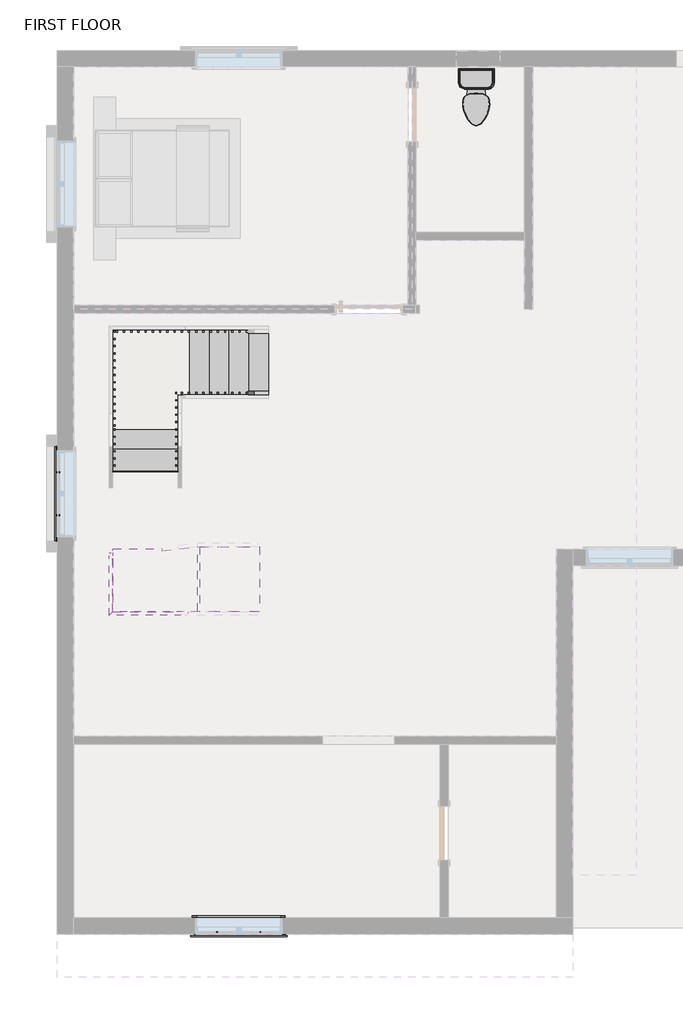
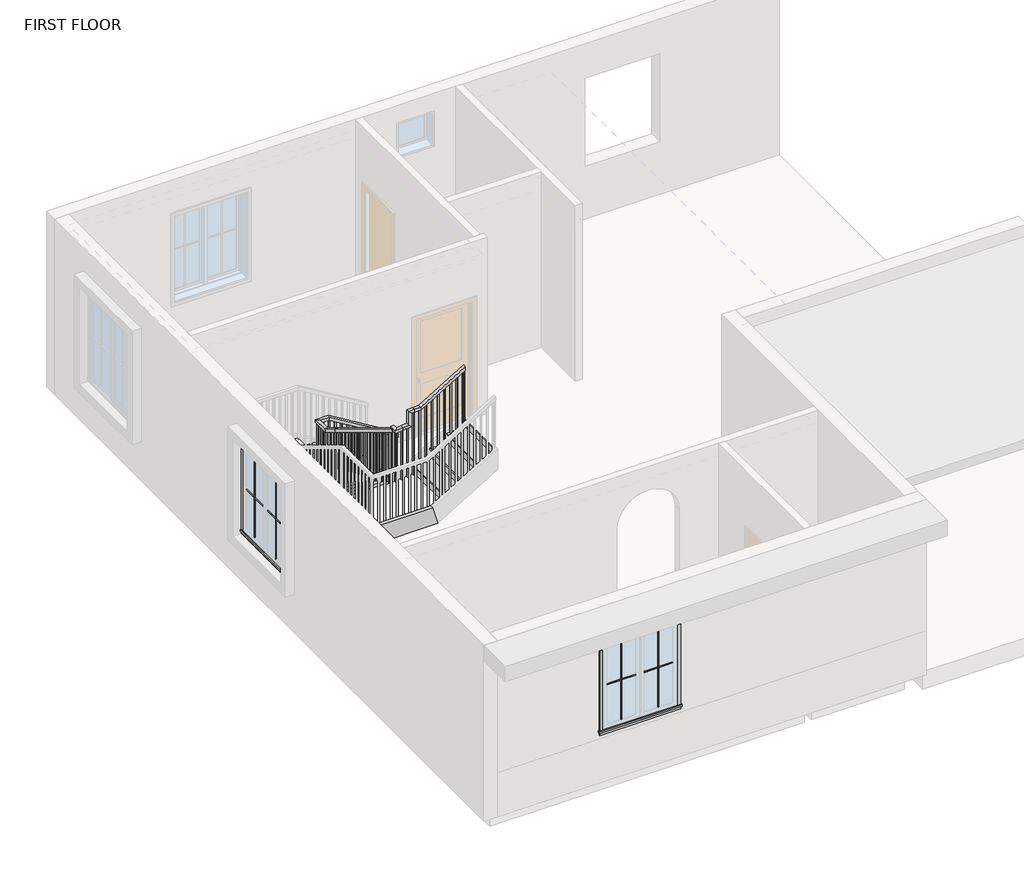
# One storey, part 3 of 4: 7 proxies, 3 stair flights, 2 members, 2 slabs, 1 flow terminal, 1 railing.
"""IFC4 building model written with IfcOpenShell, lengths in millimetres."""

from ifc_helpers import new_model, si_unit, frame, origin, place, context, project, spatial, polyline, outline, extrude, faceted_brep, transform, mapped, element, save
from components import muntin_pattern_2x2_muntin_pattern_2x2_6dad3731, muntin_pattern_2x2_muntin_pattern_2x2_a30a3345, trim_window_exterior_flat_with_sill_92b9b949, trim_window_interior_flat_picture_frame_3bb882cf, toilet_domestic_3d_toilet_domestic_3d_ba6479b0, toilet_domestic_3d_toilet_domestic_3d_30431060, non_monolithic_landing_30da2899, non_monolithic_landing_a4a5f0de, stair_flight_f80b6bc8, stair_flight_52aa9efe, stair_flight_812e3324

model = new_model("IFC4")

# Units and contexts
model_context = context("Model", 3, world=origin())
ifc_project = project(units=[si_unit("LENGTHUNIT", "METRE", prefix="MILLI")], contexts=[model_context])

# Site, building, storey
site = spatial("IfcSite", under=ifc_project)
building = spatial("IfcBuilding", under=site)
storey = spatial("IfcBuildingStorey", under=building, Name="FIRST FLOOR", Elevation=3352.8)

# Proxies
placement = place(None, origin())
muntin_pattern_2x2_muntin_pattern_2x2_shape = muntin_pattern_2x2_muntin_pattern_2x2_6dad3731(model_context)
element("IfcBuildingElementProxy", 1, Name="Muntin Pattern_2x2 : Muntin Pattern_2x2", ObjectType="Muntin Pattern_2x2 : Muntin Pattern_2x2", at=placement, inside=storey, context=model_context, shape_type="MappedRepresentation", body=[
    mapped(muntin_pattern_2x2_muntin_pattern_2x2_shape, transform((-9193.7461008, -7440.4594117, 4337.05), x_axis=(-1.0, 0.0, 0.0), y_axis=(0.0, -1.0, 0.0), z_axis=(0.0, 0.0, 1.0))),
])
element("IfcBuildingElementProxy", 2, Name="Muntin Pattern_2x2 : Muntin Pattern_2x2", ObjectType="Muntin Pattern_2x2 : Muntin Pattern_2x2", at=placement, inside=storey, context=model_context, shape_type="MappedRepresentation", body=[
    mapped(muntin_pattern_2x2_muntin_pattern_2x2_shape, transform((-12040.1336008, -1561.9469117, 4337.05), x_axis=(0.0, 1.0, 0.0), y_axis=(-1.0, 0.0, 0.0), z_axis=(0.0, 0.0, 1.0))),
])
muntin_pattern_2x2_muntin_pattern_2x2_2_shape = muntin_pattern_2x2_muntin_pattern_2x2_a30a3345(model_context)
element("IfcBuildingElementProxy", 3, Name="Muntin Pattern_2x2 : Muntin Pattern_2x2", ObjectType="Muntin Pattern_2x2 : Muntin Pattern_2x2", at=placement, inside=storey, context=model_context, shape_type="MappedRepresentation", body=[
    mapped(muntin_pattern_2x2_muntin_pattern_2x2_2_shape, transform((-9800.1711008, -7440.4594117, 4337.05), x_axis=(1.0, 0.0, 0.0), y_axis=(0.0, 1.0, 0.0), z_axis=(0.0, 0.0, 1.0))),
])
element("IfcBuildingElementProxy", 4, Name="Muntin Pattern_2x2 : Muntin Pattern_2x2", ObjectType="Muntin Pattern_2x2 : Muntin Pattern_2x2", at=placement, inside=storey, context=model_context, shape_type="MappedRepresentation", body=[
    mapped(muntin_pattern_2x2_muntin_pattern_2x2_2_shape, transform((-12040.1336008, -955.5219117, 4337.05), x_axis=(0.0, -1.0, 0.0), y_axis=(1.0, 0.0, 0.0), z_axis=(0.0, 0.0, 1.0))),
])
trim_window_exterior_flat_with_sill_shape = trim_window_exterior_flat_with_sill_92b9b949(model_context)
element("IfcBuildingElementProxy", 5, Name="Trim-Window-Exterior-Flat : with Sill", ObjectType="Trim-Window-Exterior-Flat : with Sill", at=placement, inside=storey, context=model_context, shape_type="MappedRepresentation", body=[
    mapped(trim_window_exterior_flat_with_sill_shape, transform((-9496.9586008, -7449.9844117, 5791.2), x_axis=(1.0, 0.0, 0.0), y_axis=(0.0, 0.0, 1.0), z_axis=(0.0, -1.0, 0.0))),
])
element("IfcBuildingElementProxy", 6, Name="Trim-Window-Exterior-Flat : with Sill", ObjectType="Trim-Window-Exterior-Flat : with Sill", at=placement, inside=storey, context=model_context, shape_type="MappedRepresentation", body=[
    mapped(trim_window_exterior_flat_with_sill_shape, transform((-12049.6586008, -1258.7344117, 5791.2), x_axis=(0.0, -1.0, 0.0), y_axis=(0.0, 0.0, 1.0), z_axis=(-1.0, 0.0, 0.0))),
])
trim_window_interior_flat_picture_frame_shape = trim_window_interior_flat_picture_frame_3bb882cf(model_context)
element("IfcBuildingElementProxy", 7, Name="Trim-Window-Interior-Flat : Picture Frame", ObjectType="Trim-Window-Interior-Flat : Picture Frame", at=placement, inside=storey, context=model_context, shape_type="MappedRepresentation", body=[
    mapped(trim_window_interior_flat_picture_frame_shape, transform((-9496.9586008, -7221.3844117, 5791.2), x_axis=(-1.0, 0.0, 0.0), y_axis=(0.0, 0.0, 1.0), z_axis=(0.0, 1.0, 0.0))),
])

# Flow terminal
toilet_domestic_3d_toilet_domestic_3d_shape = toilet_domestic_3d_toilet_domestic_3d_ba6479b0(model_context)
toilet_domestic_3d_toilet_domestic_3d_2_shape = toilet_domestic_3d_toilet_domestic_3d_30431060(model_context)
element("IfcFlowTerminal", 8, ObjectType="Toilet-Domestic-3D : Toilet-Domestic-3D", at=placement, inside=storey, context=model_context, shape_type="MappedRepresentation", body=[
    mapped(toilet_domestic_3d_toilet_domestic_3d_shape, transform((-6156.8586008, 4221.3155883, 3352.8), x_axis=(1.0, 0.0, 0.0), y_axis=(0.0, 1.0, 0.0), z_axis=(0.0, 0.0, 1.0))),
    mapped(toilet_domestic_3d_toilet_domestic_3d_2_shape, transform((-6156.8586008, 4221.3155883, 3352.8), x_axis=(1.0, 0.0, 0.0), y_axis=(0.0, 1.0, 0.0), z_axis=(0.0, 0.0, 1.0))),
])

# Members
element("IfcMember", 9, ObjectType="Stringer - 2\" Width", at=placement, inside=storey, context=model_context, shape_type="Brep", body=[
    faceted_brep([(-11268.1522729, -2087.9404207, 5461.0), (-11318.9522729, -2087.9404207, 5461.0), (-11318.9522729, -2966.8844117, 5461.0), (-11268.1522729, -2916.0844117, 5461.0), (-11268.1522729, -2173.0948772, 5156.2), (-11268.1522729, -2916.0844117, 5156.2), (-11318.9522729, -2173.0948772, 5156.2), (-11318.9522729, -2966.8844117, 5156.2)], [[[0, 1, 2, 3]], [[4, 0, 3, 5]], [[6, 4, 5, 7]], [[1, 6, 7, 2]], [[1, 0, 4, 6]], [[2, 7, 5, 3]]]),
])
element("IfcMember", 10, ObjectType="Stringer - 2\" Width", at=placement, inside=storey, context=model_context, shape_type="Brep", body=[
    faceted_brep([(-11268.1522729, -2916.0844117, 5461.0), (-11318.9522729, -2966.8844117, 5461.0), (-10298.6112176, -2966.8844117, 5461.0), (-10298.6112176, -2916.0844117, 5461.0), (-11268.1522729, -2916.0844117, 5156.2), (-10213.4567611, -2916.0844117, 5156.2), (-11318.9522729, -2966.8844117, 5156.2), (-10213.4567611, -2966.8844117, 5156.2)], [[[0, 1, 2, 3]], [[4, 0, 3, 5]], [[6, 4, 5, 7]], [[1, 6, 7, 2]], [[1, 0, 4, 6]], [[2, 7, 5, 3]]]),
])

# Railing
element("IfcRailing", 11, ObjectType="Handrail - Rectangular", at=placement, inside=storey, context=model_context, shape_type="SolidModel", body=[
    faceted_brep([(-9079.7156858, 130.7115003, 4436.5333333), (-9079.7156858, 130.7115003, 4377.1318731), (-9079.7156858, 181.5115003, 4377.1318731), (-9079.7156858, 181.5115003, 4436.5333333), (-10197.3156858, 130.7115003, 5113.8666667), (-10211.5080953, 130.7115003, 5063.0666667), (-10211.5080953, 181.5115003, 5063.0666667), (-10197.3156858, 181.5115003, 5113.8666667), (-10353.7522729, 130.7115003, 5113.8666667), (-10353.7522729, 130.7115003, 5063.0666667), (-10404.5522729, 181.5115003, 5063.0666667), (-10404.5522729, 181.5115003, 5113.8666667), (-10353.7522729, -76.9993654, 5113.8666667), (-10353.7522729, -91.1917748, 5063.0666667), (-10404.5522729, -91.1917748, 5063.0666667), (-10404.5522729, -76.9993654, 5113.8666667), (-10353.7522729, -356.3993654, 5283.2), (-10353.7522729, -382.7290926, 5239.7559502), (-10404.5522729, -382.7290926, 5239.7559502), (-10404.5522729, -356.3993654, 5283.2), (-10353.7522729, -1959.5850154, 6254.8276667), (-10353.7522729, -2010.3850154, 6226.2140852), (-10404.5522729, -2010.3850154, 6226.2140852), (-10404.5522729, -1959.5850154, 6254.8276667), (-10353.7522729, -1959.5850154, 6299.2), (-10353.7522729, -2010.3850154, 6248.4), (-10404.5522729, -2010.3850154, 6248.4), (-10404.5522729, -1959.5850154, 6299.2), (-10353.7522729, -2032.7993654, 6299.2), (-10353.7522729, -2032.7993654, 6248.4), (-10404.5522729, -2089.5706654, 6248.4), (-10404.5522729, -2089.5706654, 6299.2), (-10280.987739, -2024.6960544, 6299.2), (-10280.987739, -2024.6960544, 6248.4), (-10275.3652319, -2075.1839481, 6248.4), (-10275.3652319, -2075.1839481, 6299.2), (-10176.7293559, -2013.085479, 6299.2), (-10126.2414621, -2007.4629719, 6248.4), (-10120.6189551, -2057.9508656, 6248.4), (-10171.1068488, -2063.5733727, 6299.2), (-10176.7293559, -2013.085479, 6530.9636109), (-10126.2414621, -2007.4629719, 6480.1636109), (-10120.6189551, -2057.9508656, 6480.1636109), (-10171.1068488, -2063.5733727, 6530.9636109), (-10074.3522729, -2001.6844117, 6530.9636109), (-10074.3522729, -2001.6844117, 6480.1636109), (-10071.5323568, -2052.4844117, 6480.1636109), (-10071.5323568, -2052.4844117, 6530.9636109), (-9971.3423149, -2001.6844117, 6530.9636109), (-9957.1499054, -2001.6844117, 6480.1636109), (-9957.1499054, -2052.4844117, 6480.1636109), (-9971.3423149, -2052.4844117, 6530.9636109), (-9236.1522729, -2001.6844117, 6976.5333333), (-9236.1522729, -2052.4844117, 6976.5333333), (-9236.1522729, -2052.4844117, 6917.1318731), (-9236.1522729, -2001.6844117, 6917.1318731)], [[[0, 1, 2, 3]], [[1, 0, 4, 5]], [[2, 1, 5, 6]], [[3, 2, 6, 7]], [[0, 3, 7, 4]], [[5, 4, 8, 9]], [[6, 5, 9, 10]], [[7, 6, 10, 11]], [[4, 7, 11, 8]], [[9, 8, 12, 13]], [[10, 9, 13, 14]], [[11, 10, 14, 15]], [[8, 11, 15, 12]], [[13, 12, 16, 17]], [[14, 13, 17, 18]], [[15, 14, 18, 19]], [[12, 15, 19, 16]], [[17, 16, 20, 21]], [[18, 17, 21, 22]], [[19, 18, 22, 23]], [[16, 19, 23, 20]], [[21, 20, 24, 25]], [[22, 21, 25, 26]], [[23, 22, 26, 27]], [[20, 23, 27, 24]], [[25, 24, 28, 29]], [[26, 25, 29, 30]], [[27, 26, 30, 31]], [[24, 27, 31, 28]], [[29, 28, 32, 33]], [[30, 29, 33, 34]], [[31, 30, 34, 35]], [[28, 31, 35, 32]], [[33, 32, 36, 37]], [[34, 33, 37, 38]], [[35, 34, 38, 39]], [[32, 35, 39, 36]], [[37, 36, 40, 41]], [[38, 37, 41, 42]], [[39, 38, 42, 43]], [[36, 39, 43, 40]], [[41, 40, 44, 45]], [[42, 41, 45, 46]], [[43, 42, 46, 47]], [[40, 43, 47, 44]], [[45, 44, 48, 49]], [[46, 45, 49, 50]], [[47, 46, 50, 51]], [[44, 47, 51, 48]], [[52, 53, 54, 55]], [[49, 48, 52, 55]], [[50, 49, 55, 54]], [[51, 50, 54, 53]], [[48, 51, 53, 52]]]),
    extrude(outline(polyline([(6896.8197264, -9269.6673149), (5892.8, -9269.6673149), (5892.8, -9250.6173149), (6908.365181, -9250.6173149), (6896.8197264, -9269.6673149)])), frame((0.0, -2036.6094117, 0.0), z_axis=(0.0, 1.0, 0.0), x_axis=(0.0, 0.0, 1.0)), (0.0, 0.0, 1.0), 19.05),
    extrude(outline(polyline([(6835.2439689, -9371.2673149), (5892.8, -9371.2673149), (5892.8, -9352.2173149), (6846.7894234, -9352.2173149), (6835.2439689, -9371.2673149)])), frame((0.0, -2036.6094117, 0.0), z_axis=(0.0, 1.0, 0.0), x_axis=(0.0, 0.0, 1.0)), (0.0, 0.0, 1.0), 19.05),
    extrude(outline(polyline([(6773.6682113, -9472.8673149), (5892.8, -9472.8673149), (5892.8, -9453.8173149), (6785.2136658, -9453.8173149), (6773.6682113, -9472.8673149)])), frame((0.0, -2036.6094117, 0.0), z_axis=(0.0, 1.0, 0.0), x_axis=(0.0, 0.0, 1.0)), (0.0, 0.0, 1.0), 19.05),
    extrude(outline(polyline([(6712.0924537, -9574.4673149), (5723.4666667, -9574.4673149), (5723.4666667, -9555.4173149), (6723.6379083, -9555.4173149), (6712.0924537, -9574.4673149)])), frame((0.0, -2036.6094117, 0.0), z_axis=(0.0, 1.0, 0.0), x_axis=(0.0, 0.0, 1.0)), (0.0, 0.0, 1.0), 19.05),
    extrude(outline(polyline([(6650.5166961, -9676.0673149), (5723.4666667, -9676.0673149), (5723.4666667, -9657.0173149), (6662.0621507, -9657.0173149), (6650.5166961, -9676.0673149)])), frame((0.0, -2036.6094117, 0.0), z_axis=(0.0, 1.0, 0.0), x_axis=(0.0, 0.0, 1.0)), (0.0, 0.0, 1.0), 19.05),
    extrude(outline(polyline([(6588.9409386, -9777.6673149), (5723.4666667, -9777.6673149), (5723.4666667, -9758.6173149), (6600.4863931, -9758.6173149), (6588.9409386, -9777.6673149)])), frame((0.0, -2036.6094117, 0.0), z_axis=(0.0, 1.0, 0.0), x_axis=(0.0, 0.0, 1.0)), (0.0, 0.0, 1.0), 19.05),
    extrude(outline(polyline([(6527.365181, -9879.2673149), (5554.1333333, -9879.2673149), (5554.1333333, -9860.2173149), (6538.9106355, -9860.2173149), (6527.365181, -9879.2673149)])), frame((0.0, -2036.6094117, 0.0), z_axis=(0.0, 1.0, 0.0), x_axis=(0.0, 0.0, 1.0)), (0.0, 0.0, 1.0), 19.05),
    extrude(outline(polyline([(6465.7894234, -9980.8673149), (5554.1333333, -9980.8673149), (5554.1333333, -9961.8173149), (6477.334878, -9961.8173149), (6465.7894234, -9980.8673149)])), frame((0.0, -2036.6094117, 0.0), z_axis=(0.0, 1.0, 0.0), x_axis=(0.0, 0.0, 1.0)), (0.0, 0.0, 1.0), 19.05),
    extrude(outline(polyline([(-10086.7456106, -2019.0377129), (-10067.8126505, -2016.9292728), (-10065.7042103, -2035.8622329), (-10084.6371705, -2037.9706731), (-10086.7456106, -2019.0377129)])), frame((0.0, 0.0, 5384.8), z_axis=(0.0, 0.0, 1.0), x_axis=(1.0, 0.0, 0.0)), (0.0, 0.0, 1.0), 1095.3636109),
    extrude(outline(polyline([(-10187.7213981, -2030.2827271), (-10168.7884379, -2028.1742869), (-10166.6799978, -2047.1072471), (-10185.6129579, -2049.2156872), (-10187.7213981, -2030.2827271)])), frame((0.0, 0.0, 5384.8), z_axis=(0.0, 0.0, 1.0), x_axis=(1.0, 0.0, 0.0)), (0.0, 0.0, 1.0), 863.6),
    extrude(outline(polyline([(-10288.6971856, -2041.5277412), (-10269.7642254, -2039.4193011), (-10267.6557853, -2058.3522612), (-10286.5887454, -2060.4607014), (-10288.6971856, -2041.5277412)])), frame((0.0, 0.0, 5384.8), z_axis=(0.0, 0.0, 1.0), x_axis=(1.0, 0.0, 0.0)), (0.0, 0.0, 1.0), 863.6),
    extrude(outline(polyline([(-10369.6272729, -1972.4743654), (-10369.6272729, -1991.5243654), (-10388.6772729, -1991.5243654), (-10388.6772729, -1972.4743654), (-10369.6272729, -1972.4743654)])), frame((0.0, 0.0, 5215.4666667), z_axis=(0.0, 0.0, 1.0), x_axis=(1.0, 0.0, 0.0)), (0.0, 0.0, 1.0), 1032.9333333),
    extrude(outline(polyline([(-1870.8743654, 6141.6621761), (-1870.8743654, 5215.4666667), (-1889.9243654, 5215.4666667), (-1889.9243654, 6153.2076307), (-1870.8743654, 6141.6621761)])), frame((-10388.6772729, 0.0, 0.0), z_axis=(1.0, 0.0, 0.0), x_axis=(0.0, 1.0, 0.0)), (0.0, 0.0, 1.0), 19.05),
    extrude(outline(polyline([(-1769.2743654, 6080.0864185), (-1769.2743654, 5215.4666667), (-1788.3243654, 5215.4666667), (-1788.3243654, 6091.6318731), (-1769.2743654, 6080.0864185)])), frame((-10388.6772729, 0.0, 0.0), z_axis=(1.0, 0.0, 0.0), x_axis=(0.0, 1.0, 0.0)), (0.0, 0.0, 1.0), 19.05),
    extrude(outline(polyline([(-1667.6743654, 6018.510661), (-1667.6743654, 5046.1333333), (-1686.7243654, 5046.1333333), (-1686.7243654, 6030.0561155), (-1667.6743654, 6018.510661)])), frame((-10388.6772729, 0.0, 0.0), z_axis=(1.0, 0.0, 0.0), x_axis=(0.0, 1.0, 0.0)), (0.0, 0.0, 1.0), 19.05),
    extrude(outline(polyline([(-1566.0743654, 5956.9349034), (-1566.0743654, 5046.1333333), (-1585.1243654, 5046.1333333), (-1585.1243654, 5968.4803579), (-1566.0743654, 5956.9349034)])), frame((-10388.6772729, 0.0, 0.0), z_axis=(1.0, 0.0, 0.0), x_axis=(0.0, 1.0, 0.0)), (0.0, 0.0, 1.0), 19.05),
    extrude(outline(polyline([(-1464.4743654, 5895.3591458), (-1464.4743654, 5046.1333333), (-1483.5243654, 5046.1333333), (-1483.5243654, 5906.9046004), (-1464.4743654, 5895.3591458)])), frame((-10388.6772729, 0.0, 0.0), z_axis=(1.0, 0.0, 0.0), x_axis=(0.0, 1.0, 0.0)), (0.0, 0.0, 1.0), 19.05),
    extrude(outline(polyline([(-1362.8743654, 5833.7833882), (-1362.8743654, 4876.8), (-1381.9243654, 4876.8), (-1381.9243654, 5845.3288428), (-1362.8743654, 5833.7833882)])), frame((-10388.6772729, 0.0, 0.0), z_axis=(1.0, 0.0, 0.0), x_axis=(0.0, 1.0, 0.0)), (0.0, 0.0, 1.0), 19.05),
    extrude(outline(polyline([(-1261.2743654, 5772.2076307), (-1261.2743654, 4876.8), (-1280.3243654, 4876.8), (-1280.3243654, 5783.7530852), (-1261.2743654, 5772.2076307)])), frame((-10388.6772729, 0.0, 0.0), z_axis=(1.0, 0.0, 0.0), x_axis=(0.0, 1.0, 0.0)), (0.0, 0.0, 1.0), 19.05),
    extrude(outline(polyline([(-1159.6743654, 5710.6318731), (-1159.6743654, 4707.4666667), (-1178.7243654, 4707.4666667), (-1178.7243654, 5722.1773276), (-1159.6743654, 5710.6318731)])), frame((-10388.6772729, 0.0, 0.0), z_axis=(1.0, 0.0, 0.0), x_axis=(0.0, 1.0, 0.0)), (0.0, 0.0, 1.0), 19.05),
    extrude(outline(polyline([(-1058.0743654, 5649.0561155), (-1058.0743654, 4707.4666667), (-1077.1243654, 4707.4666667), (-1077.1243654, 5660.60157), (-1058.0743654, 5649.0561155)])), frame((-10388.6772729, 0.0, 0.0), z_axis=(1.0, 0.0, 0.0), x_axis=(0.0, 1.0, 0.0)), (0.0, 0.0, 1.0), 19.05),
    extrude(outline(polyline([(-956.4743654, 5587.4803579), (-956.4743654, 4707.4666667), (-975.5243654, 4707.4666667), (-975.5243654, 5599.0258125), (-956.4743654, 5587.4803579)])), frame((-10388.6772729, 0.0, 0.0), z_axis=(1.0, 0.0, 0.0), x_axis=(0.0, 1.0, 0.0)), (0.0, 0.0, 1.0), 19.05),
    extrude(outline(polyline([(-854.8743654, 5525.9046004), (-854.8743654, 4538.1333333), (-873.9243654, 4538.1333333), (-873.9243654, 5537.4500549), (-854.8743654, 5525.9046004)])), frame((-10388.6772729, 0.0, 0.0), z_axis=(1.0, 0.0, 0.0), x_axis=(0.0, 1.0, 0.0)), (0.0, 0.0, 1.0), 19.05),
    extrude(outline(polyline([(-753.2743654, 5464.3288428), (-753.2743654, 4538.1333333), (-772.3243654, 4538.1333333), (-772.3243654, 5475.8742973), (-753.2743654, 5464.3288428)])), frame((-10388.6772729, 0.0, 0.0), z_axis=(1.0, 0.0, 0.0), x_axis=(0.0, 1.0, 0.0)), (0.0, 0.0, 1.0), 19.05),
    extrude(outline(polyline([(-651.6743654, 5402.7530852), (-651.6743654, 4538.1333333), (-670.7243654, 4538.1333333), (-670.7243654, 5414.2985397), (-651.6743654, 5402.7530852)])), frame((-10388.6772729, 0.0, 0.0), z_axis=(1.0, 0.0, 0.0), x_axis=(0.0, 1.0, 0.0)), (0.0, 0.0, 1.0), 19.05),
    extrude(outline(polyline([(-550.0743654, 5341.1773276), (-550.0743654, 4368.8), (-569.1243654, 4368.8), (-569.1243654, 5352.7227822), (-550.0743654, 5341.1773276)])), frame((-10388.6772729, 0.0, 0.0), z_axis=(1.0, 0.0, 0.0), x_axis=(0.0, 1.0, 0.0)), (0.0, 0.0, 1.0), 19.05),
    extrude(outline(polyline([(-448.4743654, 5279.60157), (-448.4743654, 4368.8), (-467.5243654, 4368.8), (-467.5243654, 5291.1470246), (-448.4743654, 5279.60157)])), frame((-10388.6772729, 0.0, 0.0), z_axis=(1.0, 0.0, 0.0), x_axis=(0.0, 1.0, 0.0)), (0.0, 0.0, 1.0), 19.05),
    extrude(outline(polyline([(-342.3634997, 5215.2919545), (-342.3634997, 4199.4666667), (-361.4134997, 4199.4666667), (-361.4134997, 5226.837409), (-342.3634997, 5215.2919545)])), frame((-10388.6772729, 0.0, 0.0), z_axis=(1.0, 0.0, 0.0), x_axis=(0.0, 1.0, 0.0)), (0.0, 0.0, 1.0), 19.05),
    extrude(outline(polyline([(-240.7634997, 5153.7161969), (-240.7634997, 4199.4666667), (-259.8134997, 4199.4666667), (-259.8134997, 5165.2616515), (-240.7634997, 5153.7161969)])), frame((-10388.6772729, 0.0, 0.0), z_axis=(1.0, 0.0, 0.0), x_axis=(0.0, 1.0, 0.0)), (0.0, 0.0, 1.0), 19.05),
    extrude(outline(polyline([(-139.1634997, 5092.1404393), (-139.1634997, 4199.4666667), (-158.2134997, 4199.4666667), (-158.2134997, 5103.6858939), (-139.1634997, 5092.1404393)])), frame((-10388.6772729, 0.0, 0.0), z_axis=(1.0, 0.0, 0.0), x_axis=(0.0, 1.0, 0.0)), (0.0, 0.0, 1.0), 19.05),
    extrude(outline(polyline([(-10369.6272729, -37.5634997), (-10369.6272729, -56.6134997), (-10388.6772729, -56.6134997), (-10388.6772729, -37.5634997), (-10369.6272729, -37.5634997)])), frame((0.0, 0.0, 4199.4666667), z_axis=(0.0, 0.0, 1.0), x_axis=(1.0, 0.0, 0.0)), (0.0, 0.0, 1.0), 863.6),
    extrude(outline(polyline([(-10369.6272729, 64.0365003), (-10369.6272729, 44.9865003), (-10388.6772729, 44.9865003), (-10388.6772729, 64.0365003), (-10369.6272729, 64.0365003)])), frame((0.0, 0.0, 4199.4666667), z_axis=(0.0, 0.0, 1.0), x_axis=(1.0, 0.0, 0.0)), (0.0, 0.0, 1.0), 863.6),
    extrude(outline(polyline([(-10289.3906858, 146.5865003), (-10308.4406858, 146.5865003), (-10308.4406858, 165.6365003), (-10289.3906858, 165.6365003), (-10289.3906858, 146.5865003)])), frame((0.0, 0.0, 4199.4666667), z_axis=(0.0, 0.0, 1.0), x_axis=(1.0, 0.0, 0.0)), (0.0, 0.0, 1.0), 863.6),
    extrude(outline(polyline([(4998.6621761, -10105.2406858), (4030.1333333, -10105.2406858), (4030.1333333, -10086.1906858), (4987.1167216, -10086.1906858), (4998.6621761, -10105.2406858)])), frame((0.0, 146.5865003, 0.0), z_axis=(0.0, 1.0, 0.0), x_axis=(0.0, 0.0, 1.0)), (0.0, 0.0, 1.0), 19.05),
    extrude(outline(polyline([(4937.0864185, -10003.6406858), (4030.1333333, -10003.6406858), (4030.1333333, -9984.5906858), (4925.540964, -9984.5906858), (4937.0864185, -10003.6406858)])), frame((0.0, 146.5865003, 0.0), z_axis=(0.0, 1.0, 0.0), x_axis=(0.0, 0.0, 1.0)), (0.0, 0.0, 1.0), 19.05),
    extrude(outline(polyline([(4875.510661, -9902.0406858), (3860.8, -9902.0406858), (3860.8, -9882.9906858), (4863.9652064, -9882.9906858), (4875.510661, -9902.0406858)])), frame((0.0, 146.5865003, 0.0), z_axis=(0.0, 1.0, 0.0), x_axis=(0.0, 0.0, 1.0)), (0.0, 0.0, 1.0), 19.05),
    extrude(outline(polyline([(4813.9349034, -9800.4406858), (3860.8, -9800.4406858), (3860.8, -9781.3906858), (4802.3894488, -9781.3906858), (4813.9349034, -9800.4406858)])), frame((0.0, 146.5865003, 0.0), z_axis=(0.0, 1.0, 0.0), x_axis=(0.0, 0.0, 1.0)), (0.0, 0.0, 1.0), 19.05),
    extrude(outline(polyline([(4752.3591458, -9698.8406858), (3860.8, -9698.8406858), (3860.8, -9679.7906858), (4740.8136913, -9679.7906858), (4752.3591458, -9698.8406858)])), frame((0.0, 146.5865003, 0.0), z_axis=(0.0, 1.0, 0.0), x_axis=(0.0, 0.0, 1.0)), (0.0, 0.0, 1.0), 19.05),
    extrude(outline(polyline([(4690.7833882, -9597.2406858), (3691.4666667, -9597.2406858), (3691.4666667, -9578.1906858), (4679.2379337, -9578.1906858), (4690.7833882, -9597.2406858)])), frame((0.0, 146.5865003, 0.0), z_axis=(0.0, 1.0, 0.0), x_axis=(0.0, 0.0, 1.0)), (0.0, 0.0, 1.0), 19.05),
    extrude(outline(polyline([(4629.2076307, -9495.6406858), (3691.4666667, -9495.6406858), (3691.4666667, -9476.5906858), (4617.6621761, -9476.5906858), (4629.2076307, -9495.6406858)])), frame((0.0, 146.5865003, 0.0), z_axis=(0.0, 1.0, 0.0), x_axis=(0.0, 0.0, 1.0)), (0.0, 0.0, 1.0), 19.05),
    extrude(outline(polyline([(4567.6318731, -9394.0406858), (3691.4666667, -9394.0406858), (3691.4666667, -9374.9906858), (4556.0864185, -9374.9906858), (4567.6318731, -9394.0406858)])), frame((0.0, 146.5865003, 0.0), z_axis=(0.0, 1.0, 0.0), x_axis=(0.0, 0.0, 1.0)), (0.0, 0.0, 1.0), 19.05),
    extrude(outline(polyline([(4506.0561155, -9292.4406858), (3522.1333333, -9292.4406858), (3522.1333333, -9273.3906858), (4494.510661, -9273.3906858), (4506.0561155, -9292.4406858)])), frame((0.0, 146.5865003, 0.0), z_axis=(0.0, 1.0, 0.0), x_axis=(0.0, 0.0, 1.0)), (0.0, 0.0, 1.0), 19.05),
    extrude(outline(polyline([(4444.4803579, -9190.8406858), (3522.1333333, -9190.8406858), (3522.1333333, -9171.7906858), (4432.9349034, -9171.7906858), (4444.4803579, -9190.8406858)])), frame((0.0, 146.5865003, 0.0), z_axis=(0.0, 1.0, 0.0), x_axis=(0.0, 0.0, 1.0)), (0.0, 0.0, 1.0), 19.05),
    extrude(outline(polyline([(-10083.463015, -2018.6721517), (-10064.5300549, -2016.5637115), (-10062.4216147, -2035.4966717), (-10081.3545749, -2037.6051118), (-10083.463015, -2018.6721517)])), frame((0.0, 0.0, 5384.8), z_axis=(0.0, 0.0, 1.0), x_axis=(1.0, 0.0, 0.0)), (0.0, 0.0, 1.0), 1095.3636109),
    extrude(outline(polyline([(-10369.6272729, -2051.6600154), (-10369.6272729, -2070.7100154), (-10388.6772729, -2070.7100154), (-10388.6772729, -2051.6600154), (-10369.6272729, -2051.6600154)])), frame((0.0, 0.0, 5384.8), z_axis=(0.0, 0.0, 1.0), x_axis=(1.0, 0.0, 0.0)), (0.0, 0.0, 1.0), 863.6),
    extrude(outline(polyline([(-346.8743654, 5218.0258125), (-346.8743654, 4199.4666667), (-365.9243654, 4199.4666667), (-365.9243654, 5229.571267), (-346.8743654, 5218.0258125)])), frame((-10388.6772729, 0.0, 0.0), z_axis=(1.0, 0.0, 0.0), x_axis=(0.0, 1.0, 0.0)), (0.0, 0.0, 1.0), 19.05),
    extrude(outline(polyline([(-10369.6272729, 146.5865003), (-10388.6772729, 146.5865003), (-10388.6772729, 165.6365003), (-10369.6272729, 165.6365003), (-10369.6272729, 146.5865003)])), frame((0.0, 0.0, 4199.4666667), z_axis=(0.0, 0.0, 1.0), x_axis=(1.0, 0.0, 0.0)), (0.0, 0.0, 1.0), 863.6),
    extrude(outline(polyline([(5060.2379337, -10206.8406858), (4199.4666667, -10206.8406858), (4199.4666667, -10187.7906858), (5048.6924791, -10187.7906858), (5060.2379337, -10206.8406858)])), frame((0.0, 146.5865003, 0.0), z_axis=(0.0, 1.0, 0.0), x_axis=(0.0, 0.0, 1.0)), (0.0, 0.0, 1.0), 19.05),
    extrude(outline(polyline([(6905.5864185, -9255.2022729), (5892.8, -9255.2022729), (5892.8, -9236.1522729), (6917.1318731, -9236.1522729), (6905.5864185, -9255.2022729)])), frame((0.0, -2036.6094117, 0.0), z_axis=(0.0, 1.0, 0.0), x_axis=(0.0, 0.0, 1.0)), (0.0, 0.0, 1.0), 19.05),
    extrude(outline(polyline([(4388.6773276, -9098.7656858), (3522.1333333, -9098.7656858), (3522.1333333, -9079.7156858), (4377.1318731, -9079.7156858), (4388.6773276, -9098.7656858)])), frame((0.0, 146.5865003, 0.0), z_axis=(0.0, 1.0, 0.0), x_axis=(0.0, 0.0, 1.0)), (0.0, 0.0, 1.0), 19.05),
])

# Slabs
non_monolithic_landing_shape = non_monolithic_landing_30da2899(model_context)
element("IfcSlab", 12, ObjectType="Non-Monolithic Landing", at=placement, inside=storey, context=model_context, shape_type="MappedRepresentation", body=[
    mapped(non_monolithic_landing_shape, transform((0.0, 0.0, 0.0), x_axis=(1.0, 0.0, 0.0), y_axis=(0.0, 1.0, 0.0), z_axis=(0.0, 0.0, 1.0))),
])
non_monolithic_landing_2_shape = non_monolithic_landing_a4a5f0de(model_context)
element("IfcSlab", 13, ObjectType="Non-Monolithic Landing", at=placement, inside=storey, context=model_context, shape_type="MappedRepresentation", body=[
    mapped(non_monolithic_landing_2_shape, transform((0.0, 0.0, 0.0), x_axis=(1.0, 0.0, 0.0), y_axis=(0.0, 1.0, 0.0), z_axis=(0.0, 0.0, 1.0))),
])

# Stair flights
stair_flight_shape = stair_flight_f80b6bc8(model_context)
element("IfcStairFlight", 14, ObjectType="2\" Tread 1\" Nosing 1/4\" Riser", at=placement, inside=storey, context=model_context, shape_type="MappedRepresentation", body=[
    mapped(stair_flight_shape, transform((0.0, 0.0, 0.0), x_axis=(1.0, 0.0, 0.0), y_axis=(0.0, 1.0, 0.0), z_axis=(0.0, 0.0, 1.0))),
])
stair_flight_2_shape = stair_flight_52aa9efe(model_context)
element("IfcStairFlight", 15, ObjectType="2\" Tread 1\" Nosing 1/4\" Riser", at=placement, inside=storey, context=model_context, shape_type="MappedRepresentation", body=[
    mapped(stair_flight_2_shape, transform((0.0, 0.0, 0.0), x_axis=(1.0, 0.0, 0.0), y_axis=(0.0, 1.0, 0.0), z_axis=(0.0, 0.0, 1.0))),
])
stair_flight_3_shape = stair_flight_812e3324(model_context)
element("IfcStairFlight", 16, ObjectType="2\" Tread 1\" Nosing 1/4\" Riser", at=placement, inside=storey, context=model_context, shape_type="MappedRepresentation", body=[
    mapped(stair_flight_3_shape, transform((0.0, 0.0, 0.0), x_axis=(1.0, 0.0, 0.0), y_axis=(0.0, 1.0, 0.0), z_axis=(0.0, 0.0, 1.0))),
])

save(model, "model.ifc")

# Revit data of these elements
# Type "Muntin Pattern_2x2 : Muntin Pattern_2x2"
#   Width [instance default] = 4' - 0"
#   Thickness = 0' - 0 1/2"
#   Height [instance default] = 4' - 0"
#   Distance = 0' - 0 3/4"
#   Interior Material [instance default] = none
#   Exterior Material [instance default] = none
#   Default Elevation = 0
# Type "Trim-Window-Exterior-Flat : with Sill"
#   Trim Width = 0' - 2 1/4"
#   Trim Thickness_Picture Frame = 0' - 1 1/4"
#   Trim Thickness_with Sill = 0' - 0 3/4"
#   Sill Thickness = 0' - 1 1/4"
#   Opening Width [instance default] = 2' - 0"
#   Opening Height [instance default] = 3' - 0"
#   Default Elevation = 4' - 0"
#   Sill = yes
#   Picture Frame = no
#   Trim Material [instance default] = none
# Type "Trim-Window-Interior-Flat : Picture Frame"
#   Trim Thickness_Picture Frame = 0' - 1 1/4"
#   Trim Width = 0' - 2 1/4"
#   Trim Thickness_with Sill = 0' - 0 3/4"
#   Sill Thickness = 0' - 1 1/4"
#   Opening Width [instance default] = 2' - 0"
#   Opening Height [instance default] = 3' - 0"
#   Default Elevation = 4' - 0"
#   Sill = no
#   Picture Frame = yes
#   Trim Material [instance default] = none
# Type "Toilet-Domestic-3D : Toilet-Domestic-3D"
#   Assembly Code = "D2010110"
#   Toilet - Bowl/Basin Material = Porcelain, Linen
#   Toilet - Seat Material = Laminate, Linen, Matte
#   Default Elevation = 0
# Type "Handrail - Rectangular"
#   Assembly Code = "C2010400"
#   built-in parameter 1008612 = 0.0416667 (stored number, unit not read)
#   built-in parameter 1008611 = 0.0416667 (stored number, unit not read)
#   built-in parameter 1008609 = 0.333333 (stored number, unit not read)
#   built-in parameter 1008604 = 0.166667 (stored number, unit not read)
#   built-in parameter 1008603 = 0.166667 (stored number, unit not read)
#   Railing Height = 3' - 0"
#   built-in parameter 1008630 = 2
#   built-in parameter 1008610 = 2
#   built-in parameter 1008618 = Baluster - Square : 3/4"
# Elements 1, 2, 3, 4 (IfcBuildingElementProxy, "Muntin Pattern_2x2 : Muntin Pattern_2x2")
#   Width = 1' - 6 5/8"
#   Height = 4' - 6 1/2"
#   Interior Material = Wood - Stained
#   Exterior Material = BLACK MATERIAL
#   Phase Created = New Construction
#   Materials on its faces: "BLACK MATERIAL", "Wood - Stained"
# Elements 5, 6 (IfcBuildingElementProxy, "Trim-Window-Exterior-Flat : with Sill")
#   Opening Width = 4' - 0"
#   Opening Height = 5' - 0"
#   Trim Material = BLACK MATERIAL
#   Phase Created = New Construction
#   Materials on its faces: "BLACK MATERIAL"
# Element 7 (IfcBuildingElementProxy, "Trim-Window-Interior-Flat : Picture Frame")
#   Opening Width = 4' - 0"
#   Opening Height = 5' - 0"
#   Trim Material = Wood - Stained
#   Phase Created = New Construction
#   Materials on its faces: "Wood - Stained"
# Element 8 (IfcFlowTerminal, "Toilet-Domestic-3D : Toilet-Domestic-3D")
#   Mark = "4"
#   Phase Created = New Construction
#   Materials on its faces: "Porcelain, Linen", "Laminate, Linen, Matte"
# Elements 9, 10 (IfcMember, "Stringer - 2\" Width")
#   Phase Created = New Construction
# Element 11 (IfcRailing, "Handrail - Rectangular")
#   Phase Created = New Construction
# Elements 12, 13 (IfcSlab, "Non-Monolithic Landing")
#   Phase Created = New Construction
# Elements 14, 15, 16 (IfcStairFlight, "2\" Tread 1\" Nosing 1/4\" Riser")
#   Phase Created = New Construction
# Materials
#   "Porcelain, Linen": class "Ceramic", colour RGB 249 239 230, transparency 0, Description = "Porcelain, linen", Cost = 0
#   "Laminate, Linen, Matte": class "Plastic", colour RGB 249 239 230, transparency 0, Description = "Plastic Laminate - Linen, Matte", Cost = 0
#   "BLACK MATERIAL": class "Generic", colour RGB 120 120 120, transparency 0, Cost = 0
#   "Wood - Stained": class "Wood", colour RGB 224 178 126, transparency 0, Cost = 0
